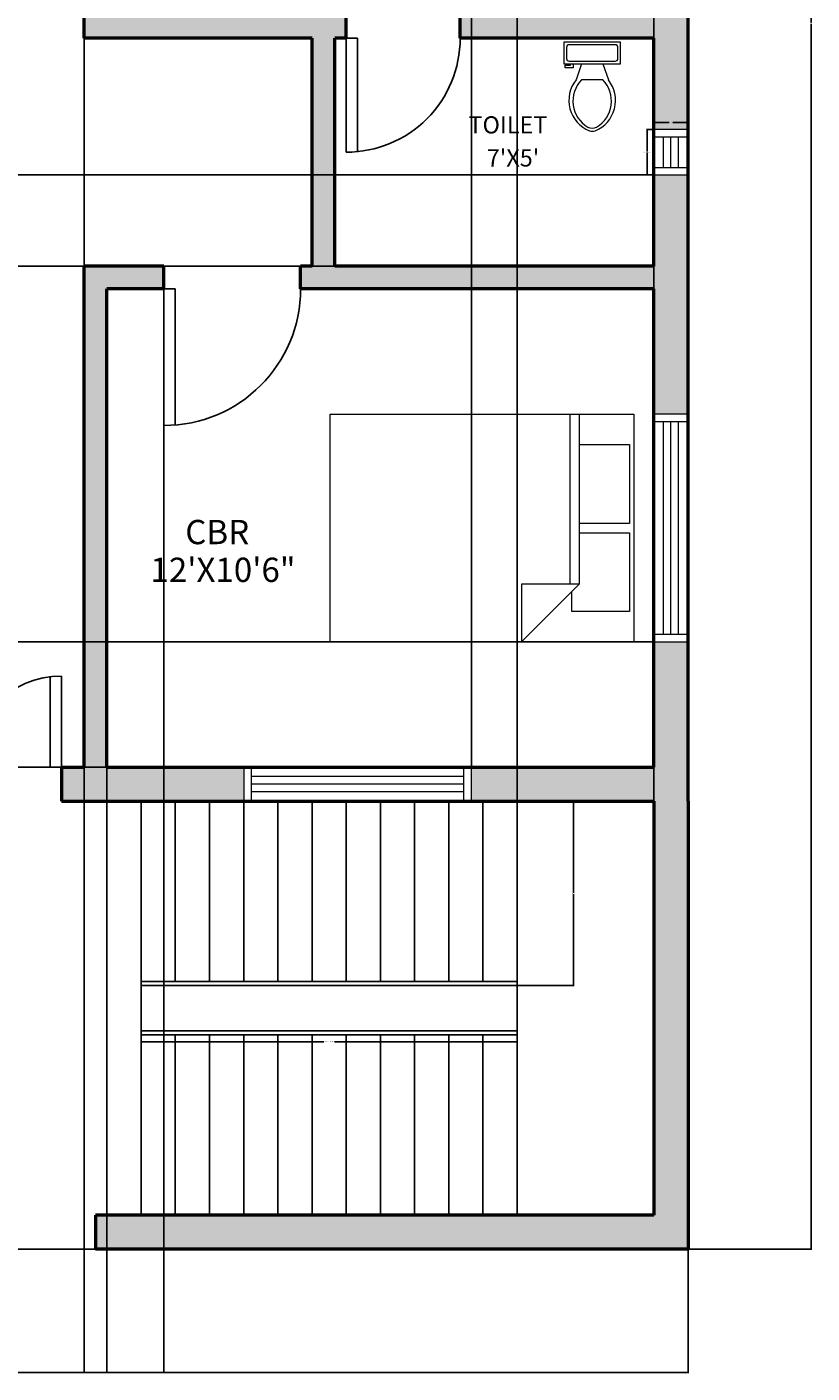
# Model space of a CAD drawing. Units: inches. Extents: x 96 to 522, y 502 to 1213.
# Tile 2 of 5: x 315 to 522, y 502 to 856. Entities that reach past the tile are written whole.
import ezdxf

# ---------------------------------------------------------------- set-up
doc = ezdxf.new("R2010")
doc.units = ezdxf.units.IN
doc.layers.get('Defpoints').update_dxf_attribs({"color": 90})
for name, color, linetype, lineweight in [('A-ANNO-DIMS', 2, 'Continuous', 18), ('A-AREA-IDEN', 7, 'Continuous', 25), ('A-DOOR', 3, 'Continuous', 25), ('A-FLOR', 7, 'Continuous', 25), ('A-FLOR-FIXT', 9, 'Continuous', 18), ('A-FLOR-STRS', 7, 'Continuous', 25), ('A-FURN', 8, 'Continuous', 18), ('A-GLAZ', 4, 'Continuous', 18), ('A-WALL', 7, 'Continuous', 50)]:
    doc.layers.add(name, color=color, linetype=linetype, lineweight=lineweight)
doc.layers.add('A-WALL-PATT', color=252, linetype='Continuous', lineweight=13, true_color=0x939598)
doc.styles.get("Standard").update_dxf_attribs({"font": 'arial.ttf'})
doc.dimstyles.get("Standard").update_dxf_attribs({"dimtxt": 0.18, "dimasz": 0.18, "dimexe": 0.18, "dimexo": 0.0625, "dimgap": 0.09, "dimtad": 0, "dimtih": 1, "dimtoh": 1, "dimdec": 4, "dimzin": 0, "dimdsep": 46, "dimtxsty": 'Standard', "dimcen": 0.09, "dimadec": 0, "dimazin": 0, "dimtfac": 1, "dimtdec": 4, "dimtofl": 0, "dimtmove": 0, "dimatfit": 3, "dimfxl": 1, "dimtolj": 1, "dimtzin": 0, "dimarcsym": 0})

# ---------------------------------------------------------------- blocks, each defined once
blk = doc.blocks.new('Bed - Queen')
for p, q in [((0, -80.00003), (0, 0)), ((0, 0), (59.99999, 0)), ((59.99999, 0), (59.99999, -80.00003)), ((7.99999, -1.2), (28.79998, -1.2)), ((7.99999, -14.4), (7.99999, -1.2)), ((28.79998, -1.2), (28.79998, -14.4)), ((31.19999, -1.2), (51.99999, -1.2)), ((31.19999, -14.4), (31.19999, -1.2)), ((51.99999, -1.2), (51.99999, -16.4)), ((0, -14.4), (44.8, -14.4)), ((44.8, -16.8), (0, -16.8)), ((59.99999, -29.6), (44.8, -14.4)), ((44.8, -14.4), (44.8, -29.6)), ((51.99999, -16.4), (46.79936, -16.4)), ((44.8, -29.6), (59.99999, -29.6)), ((59.99999, -80.00003), (0, -80.00003))]:
    blk.add_line(p, q)
blk = doc.blocks.new('Toilet - top')
for p, q in [((9.5, -6), (9.5, -2)), ((-10, -8.5), (-8, -8.5)), ((-10, -9.5), (-10, -8.5)), ((-7, -9.5), (-10, -9.5)), ((-8, -8.5), (-8, -8)), ((-7, -8), (-7, -9.5)), ((-4, -8), (-6, -14)), ((4, -8), (6, -14)), ((4, -14), (-4, -14))]:
    blk.add_line(p, q)
blk.add_lwpolyline([(10.5, -8), (10.5, 0), (-10.5, 0), (-10.5, -8)], close=True)
for points in [[(-9.5, -2), (-9.5, -6)], [(8.5, -1), (-8.5, -1)], [(-8.5, -7), (8.5, -7)]]:
    blk.add_lwpolyline(points)
for centre, radius, start, end in [((-8.62, -1.88), 0.884, 81.8699, 188.1301), ((8.62, -1.88), 0.884, 351.8699, 98.1301), ((-8.62, -6.12), 0.884, 171.8699, 278.1301), ((8.62, -6.12), 0.884, 261.8699, 8.1301), ((3.52, -21.58), 12.17, 141.4691, 247.9714), ((4.2, -21.82), 11.33, 136.3677, 238.9468), ((-3.52, -21.58), 12.17, 292.0284, 38.5307), ((-4.2, -21.82), 11.33, 301.053, 43.6321), ((0, -27.88), 4, 245.7318, 294.2682), ((0, -29), 4, 254.8605, 285.1395)]:
    blk.add_arc(centre, radius, start, end)
blk = doc.blocks.new('WIN-60IN')
for p, q in [((60, 9), (0, 9)), ((0, 9), (0, 0)), ((2, 9), (2, 0)), ((58, 0), (58, 9)), ((60, 0), (60, 9)), ((2, 6.5), (58, 6.5)), ((2, 4.5), (58, 4.5)), ((0, 0), (60, 0)), ((2, 2.5), (58, 2.5))]:
    blk.add_line(p, q)
blk = doc.blocks.new('WIN-12IN')
for p, q in [((0, 12), (0, 0)), ((9, 12), (0, 12)), ((9, 0), (9, 12)), ((9, 10), (0, 10)), ((2.5, 10), (2.5, 2)), ((4.5, 10), (4.5, 2)), ((6.5, 10), (6.5, 2)), ((0, 2), (9, 2)), ((0, 0), (9, 0))]:
    blk.add_line(p, q)
blk = doc.blocks.new('DOOR-SGL-36IN')
for p, q in [((36, 3), (0, 3)), ((0, 0), (0, 3)), ((36, 0), (0, 0))]:
    blk.add_line(p, q)
blk.add_arc((0, 0), 36, 0, 90)
blk = doc.blocks.new('DOOR-SGL-30IN')
for p, q in [((30, 30), (0, 30)), ((0, 30), (0, 27)), ((30, 27), (0, 27))]:
    blk.add_line(p, q)
blk.add_arc((0, 30), 30, 270, 0)
blk = doc.blocks.new('DOOR-DBL-48IN')
for p, q in [((0, 24), (0, 0)), ((3, 24), (3, 0)), ((45, 24), (45, 0)), ((48, 24), (48, 0)), ((0, 0), (3, 0)), ((48, 0), (45, 0))]:
    blk.add_line(p, q)
for centre, start, end in [((0, 0), 0, 90), ((48, 0), 90, 180)]:
    blk.add_arc(centre, 24, start, end)
blk = doc.blocks.new('STAIR-FLIGHT-11-TREAD')
for p, q in [((0, 48.5), (0, 0)), ((9, 48.5), (9, 1)), ((18, 48.5), (18, 1)), ((27, 48.5), (27, 1)), ((36, 48.5), (36, 1)), ((45, 48.5), (45, 1)), ((54, 48.5), (54, 1)), ((63, 48.5), (63, 1)), ((72, 48.5), (72, 1)), ((81, 48.5), (81, 1)), ((90, 48.5), (90, 1)), ((99, 48.5), (99, 1)), ((0, 1), (99, 1)), ((0, 0), (99, 0)), ((99, 0), (99, 1))]:
    blk.add_line(p, q)
blk = doc.blocks.new('*D19')
at = {"layer": 'A-ANNO-DIMS', "color": 0, "lineweight": -2, "transparency": 16777216}
for p, q in [((480.15, 829.25), (478.23, 829.25)), ((478.41, 829.07), (478.41, 823.43)), ((478.41, 817.43), (478.41, 823.07)), ((480.15, 817.25), (478.23, 817.25))]:
    blk.add_line(p, q, dxfattribs=at)
at = {"layer": 'A-ANNO-DIMS', "color": 0, "transparency": 16777216}
for points in [[(478.38, 829.07), (478.44, 829.07), (478.41, 829.25)], [(478.38, 817.43), (478.44, 817.43), (478.41, 817.25)]]:
    blk.add_solid(points, dxfattribs=at)
at = {"layer": 'Defpoints', "color": 0, "transparency": 16777216}
for p in [(480.21, 829.25), (478.41, 817.25), (480.21, 817.25)]:
    blk.add_point(p, dxfattribs=at)
at = {"layer": 'A-ANNO-DIMS', "color": 0, "transparency": 16777216, "insert": (478.41, 823.25), "char_height": 0.18, "attachment_point": 5}
blk.add_mtext('\\A1;WINDOW 12 TYP.', dxfattribs=at)
blk = doc.blocks.new('*D20')
at = {"layer": 'A-ANNO-DIMS', "color": 0, "lineweight": -2, "transparency": 16777216}
for p, q in [((480.21, 829.31), (480.21, 831.23)), ((480.39, 831.05), (484.25, 831.05)), ((489.03, 831.05), (485.17, 831.05)), ((489.21, 829.31), (489.21, 831.23))]:
    blk.add_line(p, q, dxfattribs=at)
at = {"layer": 'A-ANNO-DIMS', "color": 0, "transparency": 16777216}
for points in [[(480.39, 831.08), (480.39, 831.02), (480.21, 831.05)], [(489.03, 831.08), (489.03, 831.02), (489.21, 831.05)]]:
    blk.add_solid(points, dxfattribs=at)
at = {"layer": 'Defpoints', "color": 0, "transparency": 16777216}
for p in [(480.21, 831.05), (480.21, 829.25), (489.21, 829.25)]:
    blk.add_point(p, dxfattribs=at)
at = {"layer": 'A-ANNO-DIMS', "color": 0, "transparency": 16777216, "insert": (484.71, 831.05), "char_height": 0.18, "attachment_point": 5}
blk.add_mtext('\\A1;9 TYP.', dxfattribs=at)
blk = doc.blocks.new('*D31')
at = {"layer": 'A-ANNO-DIMS', "color": 0, "lineweight": -2, "transparency": 16777216}
for p, q in [((345.21, 603.69), (345.21, 588.72)), ((444.21, 603.69), (444.21, 588.72)), ((345.39, 588.9), (393.3, 588.9)), ((444.03, 588.9), (396.13, 588.9))]:
    blk.add_line(p, q, dxfattribs=at)
at = {"layer": 'A-ANNO-DIMS', "color": 0, "transparency": 16777216}
for points in [[(345.39, 588.93), (345.39, 588.87), (345.21, 588.9)], [(444.03, 588.93), (444.03, 588.87), (444.21, 588.9)]]:
    blk.add_solid(points, dxfattribs=at)
at = {"layer": 'Defpoints', "color": 0, "transparency": 16777216}
for p in [(345.21, 603.75), (444.21, 603.75), (444.21, 588.9)]:
    blk.add_point(p, dxfattribs=at)
at = {"layer": 'A-ANNO-DIMS', "color": 0, "transparency": 16777216, "insert": (394.71, 588.9), "char_height": 0.18, "attachment_point": 5}
blk.add_mtext('\\A1;STAIR FLIGHT 99 TYP.', dxfattribs=at)
blk = doc.blocks.new('*D32')
at = {"layer": 'A-ANNO-DIMS', "color": 0, "lineweight": -2, "transparency": 16777216}
for p, q in [((444.27, 652.25), (459.24, 652.25)), ((459.06, 652.07), (459.06, 628.18)), ((459.06, 603.93), (459.06, 627.82)), ((444.27, 603.75), (459.24, 603.75))]:
    blk.add_line(p, q, dxfattribs=at)
at = {"layer": 'A-ANNO-DIMS', "color": 0, "transparency": 16777216}
for points in [[(459.03, 652.07), (459.09, 652.07), (459.06, 652.25)], [(459.03, 603.93), (459.09, 603.93), (459.06, 603.75)]]:
    blk.add_solid(points, dxfattribs=at)
at = {"layer": 'Defpoints', "color": 0, "transparency": 16777216}
for p in [(444.21, 652.25), (459.06, 652.25), (444.21, 603.75)]:
    blk.add_point(p, dxfattribs=at)
at = {"layer": 'A-ANNO-DIMS', "color": 0, "transparency": 16777216, "insert": (459.06, 628), "char_height": 0.18, "attachment_point": 5}
blk.add_mtext('\\A1;49 TYP.', dxfattribs=at)
blk = doc.blocks.new('*D47')
at = {"layer": 'A-ANNO-DIMS', "color": 0, "lineweight": -2, "transparency": 16777216}
for p, q in [((129.21, 534.19), (129.21, 501.62)), ((489.21, 534.19), (489.21, 501.62)), ((129.39, 501.8), (308.92, 501.8)), ((489.03, 501.8), (309.5, 501.8))]:
    blk.add_line(p, q, dxfattribs=at)
at = {"layer": 'A-ANNO-DIMS', "color": 0, "transparency": 16777216}
for points in [[(129.39, 501.83), (129.39, 501.77), (129.21, 501.8)], [(489.03, 501.83), (489.03, 501.77), (489.21, 501.8)]]:
    blk.add_solid(points, dxfattribs=at)
at = {"layer": 'Defpoints', "color": 0, "transparency": 16777216}
for p in [(129.21, 534.25), (489.21, 534.25), (489.21, 501.8)]:
    blk.add_point(p, dxfattribs=at)
at = {"layer": 'A-ANNO-DIMS', "color": 0, "transparency": 16777216, "insert": (309.21, 501.8), "char_height": 0.18, "attachment_point": 5}
blk.add_mtext('\\A1;360', dxfattribs=at)
blk = doc.blocks.new('*D48')
at = {"layer": 'A-ANNO-DIMS', "color": 0, "lineweight": -2, "transparency": 16777216}
for p, q in [((335.27, 1180.25), (521.84, 1180.25)), ((521.66, 1180.07), (521.66, 857.43)), ((521.66, 534.43), (521.66, 857.07)), ((489.27, 534.25), (521.84, 534.25))]:
    blk.add_line(p, q, dxfattribs=at)
at = {"layer": 'A-ANNO-DIMS', "color": 0, "transparency": 16777216}
for points in [[(521.63, 1180.07), (521.69, 1180.07), (521.66, 1180.25)], [(521.63, 534.43), (521.69, 534.43), (521.66, 534.25)]]:
    blk.add_solid(points, dxfattribs=at)
at = {"layer": 'Defpoints', "color": 0, "transparency": 16777216}
for p in [(335.21, 1180.25), (521.66, 1180.25), (489.21, 534.25)]:
    blk.add_point(p, dxfattribs=at)
at = {"layer": 'A-ANNO-DIMS', "color": 0, "transparency": 16777216, "insert": (521.66, 857.25), "char_height": 0.18, "attachment_point": 5}
blk.add_mtext('\\A1;646', dxfattribs=at)
blk = doc.blocks.new('*D55')
at = {"layer": 'A-ANNO-DIMS', "color": 0, "lineweight": -2, "transparency": 16777216}
for p, q in [((432.21, 661.31), (432.21, 1212.88)), ((480.21, 661.31), (480.21, 1212.88)), ((432.39, 1212.7), (455.99, 1212.7)), ((480.03, 1212.7), (456.43, 1212.7))]:
    blk.add_line(p, q, dxfattribs=at)
at = {"layer": 'A-ANNO-DIMS', "color": 0, "transparency": 16777216}
for points in [[(432.39, 1212.73), (432.39, 1212.67), (432.21, 1212.7)], [(480.03, 1212.73), (480.03, 1212.67), (480.21, 1212.7)]]:
    blk.add_solid(points, dxfattribs=at)
at = {"layer": 'Defpoints', "color": 0, "transparency": 16777216}
for p in [(480.21, 1212.7), (432.21, 661.25), (480.21, 661.25)]:
    blk.add_point(p, dxfattribs=at)
at = {"layer": 'A-ANNO-DIMS', "color": 0, "transparency": 16777216, "insert": (456.21, 1212.7), "char_height": 0.18, "attachment_point": 5}
blk.add_mtext('\\A1;48', dxfattribs=at)
blk = doc.blocks.new('*D60')
at = {"layer": 'A-ANNO-DIMS', "color": 0, "lineweight": -2, "transparency": 16777216}
for p, q in [((480.15, 694.25), (96.58, 694.25)), ((96.76, 694.07), (96.76, 677.93)), ((96.76, 661.43), (96.76, 677.57)), ((480.15, 661.25), (96.58, 661.25))]:
    blk.add_line(p, q, dxfattribs=at)
at = {"layer": 'A-ANNO-DIMS', "color": 0, "transparency": 16777216}
for points in [[(96.73, 694.07), (96.79, 694.07), (96.76, 694.25)], [(96.73, 661.43), (96.79, 661.43), (96.76, 661.25)]]:
    blk.add_solid(points, dxfattribs=at)
at = {"layer": 'Defpoints', "color": 0, "transparency": 16777216}
for p in [(96.76, 694.25), (480.21, 694.25), (480.21, 661.25)]:
    blk.add_point(p, dxfattribs=at)
at = {"layer": 'A-ANNO-DIMS', "color": 0, "transparency": 16777216, "insert": (96.76, 677.75), "char_height": 0.18, "attachment_point": 5}
blk.add_mtext('\\A1;33', dxfattribs=at)
blk = doc.blocks.new('*D61')
at = {"layer": 'A-ANNO-DIMS', "color": 0, "lineweight": -2, "transparency": 16777216}
for p, q in [((480.15, 817.25), (96.58, 817.25)), ((96.76, 817.07), (96.76, 805.43)), ((96.76, 793.43), (96.76, 805.07)), ((480.15, 793.25), (96.58, 793.25))]:
    blk.add_line(p, q, dxfattribs=at)
at = {"layer": 'A-ANNO-DIMS', "color": 0, "transparency": 16777216}
for points in [[(96.73, 817.07), (96.79, 817.07), (96.76, 817.25)], [(96.73, 793.43), (96.79, 793.43), (96.76, 793.25)]]:
    blk.add_solid(points, dxfattribs=at)
at = {"layer": 'Defpoints', "color": 0, "transparency": 16777216}
for p in [(96.76, 817.25), (480.21, 817.25), (480.21, 793.25)]:
    blk.add_point(p, dxfattribs=at)
at = {"layer": 'A-ANNO-DIMS', "color": 0, "transparency": 16777216, "insert": (96.76, 805.25), "char_height": 0.18, "attachment_point": 5}
blk.add_mtext('\\A1;24', dxfattribs=at)
blk = doc.blocks.new('*D65')
at = {"layer": 'A-ANNO-DIMS', "color": 0, "lineweight": -2, "transparency": 16777216}
for p, q in [((444.21, 543.31), (444.21, 1212.88)), ((480.21, 543.31), (480.21, 1212.88)), ((444.39, 1212.7), (461.99, 1212.7)), ((480.03, 1212.7), (462.43, 1212.7))]:
    blk.add_line(p, q, dxfattribs=at)
at = {"layer": 'A-ANNO-DIMS', "color": 0, "transparency": 16777216}
for points in [[(444.39, 1212.73), (444.39, 1212.67), (444.21, 1212.7)], [(480.03, 1212.73), (480.03, 1212.67), (480.21, 1212.7)]]:
    blk.add_solid(points, dxfattribs=at)
at = {"layer": 'Defpoints', "color": 0, "transparency": 16777216}
for p in [(480.21, 1212.7), (444.21, 543.25), (480.21, 543.25)]:
    blk.add_point(p, dxfattribs=at)
at = {"layer": 'A-ANNO-DIMS', "color": 0, "transparency": 16777216, "insert": (462.21, 1212.7), "char_height": 0.18, "attachment_point": 5}
blk.add_mtext('\\A1;36', dxfattribs=at)
blk = doc.blocks.new('*D66')
at = {"layer": 'A-ANNO-DIMS', "color": 0, "lineweight": -2, "transparency": 16777216}
for p, q in [((330.21, 1033.19), (330.21, 501.62)), ((276.21, 997.19), (276.21, 501.62)), ((276.39, 501.8), (302.99, 501.8)), ((330.03, 501.8), (303.43, 501.8))]:
    blk.add_line(p, q, dxfattribs=at)
at = {"layer": 'A-ANNO-DIMS', "color": 0, "transparency": 16777216}
for points in [[(276.39, 501.83), (276.39, 501.77), (276.21, 501.8)], [(330.03, 501.83), (330.03, 501.77), (330.21, 501.8)]]:
    blk.add_solid(points, dxfattribs=at)
at = {"layer": 'Defpoints', "color": 0, "transparency": 16777216}
for p in [(330.21, 1033.25), (276.21, 997.25), (330.21, 501.8)]:
    blk.add_point(p, dxfattribs=at)
at = {"layer": 'A-ANNO-DIMS', "color": 0, "transparency": 16777216, "insert": (303.21, 501.8), "char_height": 0.18, "attachment_point": 5}
blk.add_mtext('\\A1;54', dxfattribs=at)
blk = doc.blocks.new('*D70')
at = {"layer": 'A-ANNO-DIMS', "color": 0, "lineweight": -2, "transparency": 16777216}
for p, q in [((336.21, 787.19), (336.21, 501.62)), ((351.21, 787.19), (351.21, 501.62)), ((336.39, 501.8), (343.5, 501.8)), ((351.03, 501.8), (343.92, 501.8))]:
    blk.add_line(p, q, dxfattribs=at)
at = {"layer": 'A-ANNO-DIMS', "color": 0, "transparency": 16777216}
for points in [[(336.39, 501.83), (336.39, 501.77), (336.21, 501.8)], [(351.03, 501.83), (351.03, 501.77), (351.21, 501.8)]]:
    blk.add_solid(points, dxfattribs=at)
at = {"layer": 'Defpoints', "color": 0, "transparency": 16777216}
for p in [(336.21, 787.25), (351.21, 787.25), (351.21, 501.8)]:
    blk.add_point(p, dxfattribs=at)
at = {"layer": 'A-ANNO-DIMS', "color": 0, "transparency": 16777216, "insert": (343.71, 501.8), "char_height": 0.18, "attachment_point": 5}
blk.add_mtext('\\A1;15', dxfattribs=at)

msp = doc.modelspace()

# ---------------------------------------------------------------- hatches: boundary and pattern name
at = {"layer": 'A-WALL-PATT'}
h = msp.add_hatch(color=256, dxfattribs=at)
h.dxf.hatch_style = 1
h.paths.add_polyline_path([(174.2111, 1156.2511), (129.2111, 1156.2511), (129.2111, 1105.2511), (138.2111, 1105.2511), (138.2111, 1147.2511), (174.2111, 1147.2511)])
h.paths.add_polyline_path([(287.2111, 1156.2511), (234.2111, 1156.2511), (234.2111, 1147.2511), (270.2111, 1147.2511), (270.2111, 1003.2511), (267.2111, 1003.2511), (267.2111, 997.2511), (276.2111, 997.2511), (276.2111, 1147.2511), (287.2111, 1147.2511)])
h.paths.add_polyline_path([(342.2111, 1156.2511), (335.2111, 1156.2511), (335.2111, 1147.2511), (338.2111, 1147.2511), (338.2111, 1081.2511), (342.2111, 1081.2511), (342.2111, 1147.2511)])
h.paths.add_polyline_path([(489.2111, 1156.2511), (402.2111, 1156.2511), (402.2111, 1147.2511), (402.2111, 1141.2511), (408.2111, 1141.2511), (408.2111, 1147.2511), (480.2111, 1147.2511), (480.2111, 1123.2511), (489.2111, 1123.2511)])
h.paths.add_polyline_path([(489.2111, 1111.2511), (480.2111, 1111.2511), (480.2111, 1087.2511), (408.2111, 1087.2511), (408.2111, 1111.2511), (402.2111, 1111.2511), (402.2111, 1066.2511), (408.2111, 1066.2511), (408.2111, 1081.2511), (480.2111, 1081.2511), (480.2111, 1063.2511), (489.2111, 1063.2511)])
h.paths.add_polyline_path([(489.2111, 1051.2511), (480.2111, 1051.2511), (480.2111, 1033.2511), (408.2111, 1033.2511), (408.2111, 1036.2511), (402.2111, 1036.2511), (402.2111, 1033.2511), (338.2111, 1033.2511), (330.2111, 1033.2511), (330.2111, 923.2511), (336.2111, 923.2511), (336.2111, 1027.2511), (338.2111, 1027.2511), (402.2111, 1027.2511), (480.2111, 1027.2511), (480.2111, 973.2511), (489.2111, 973.2511)])
h.paths.add_polyline_path([(489.2111, 913.2511), (480.2111, 913.2511), (480.2111, 859.2511), (429.2111, 859.2511), (429.2111, 853.2511), (480.2111, 853.2511), (480.2111, 829.2511), (489.2111, 829.2511)])
h.paths.add_polyline_path([(489.2111, 817.2511), (480.2111, 817.2511), (480.2111, 793.2511), (402.2111, 793.2511), (396.2111, 793.2511), (396.2111, 853.2511), (399.2111, 853.2511), (399.2111, 859.2511), (338.2111, 859.2511), (336.2111, 859.2511), (336.2111, 877.2511), (336.2111, 883.2511), (336.2111, 887.2511), (330.2111, 887.2511), (330.2111, 883.2511), (326.2111, 883.2511), (326.2111, 877.2511), (330.2111, 877.2511), (330.2111, 853.2511), (338.2111, 853.2511), (390.2111, 853.2511), (390.2111, 793.2511), (387.2111, 793.2511), (387.2111, 787.2511), (402.2111, 787.2511), (480.2111, 787.2511), (480.2111, 754.2511), (489.2111, 754.2511)])
h.paths.add_polyline_path([(489.2111, 694.2511), (480.2111, 694.2511), (480.2111, 661.2511), (432.2111, 661.2511), (432.2111, 652.2511), (480.2111, 652.2511), (480.2111, 543.2511), (333.2111, 543.2511), (333.2111, 534.2511), (489.2111, 534.2511), (489.2111, 652.2511)])
h.paths.add_polyline_path([(372.2111, 661.2511), (336.2111, 661.2511), (336.2111, 787.2511), (338.2111, 787.2511), (351.2111, 787.2511), (351.2111, 793.2511), (338.2111, 793.2511), (330.2111, 793.2511), (330.2111, 661.2511), (324.2111, 661.2511), (324.2111, 652.2511), (372.2111, 652.2511)])
h.paths.add_polyline_path([(138.2111, 680.6946), (129.2111, 680.6946), (129.2111, 652.2511), (177.2111, 652.2511), (177.2111, 661.2511), (138.2111, 661.2511)])
h.paths.add_polyline_path([(276.2111, 661.2511), (237.2111, 661.2511), (237.2111, 652.2511), (276.2111, 652.2511)])
h.paths.add_polyline_path([(138.2111, 803.1393), (129.2111, 803.1393), (129.2111, 740.6946), (138.2111, 740.6946)])
h.paths.add_polyline_path([(138.2111, 907.2511), (129.2111, 907.2511), (129.2111, 863.1393), (138.2111, 863.1393), (138.2111, 877.2511), (276.2111, 877.2511), (276.2111, 883.2511), (204.2111, 883.2511), (204.2111, 886.2511), (198.2111, 886.2511), (198.2111, 883.2511), (138.2111, 883.2511)])
h.paths.add_polyline_path([(138.2111, 943.2511), (198.2111, 943.2511), (198.2111, 916.2511), (204.2111, 916.2511), (204.2111, 949.2511), (138.2111, 949.2511), (138.2111, 997.2511), (231.2111, 997.2511), (231.2111, 1003.2511), (138.2111, 1003.2511), (138.2111, 1045.2511), (129.2111, 1045.2511), (129.2111, 919.2511), (138.2111, 919.2511)])

# ---------------------------------------------------------------- linework, layer by layer
at = {"layer": 'A-FLOR'}
msp.add_line((129.2111, 534.2511), (333.2111, 534.2511), dxfattribs=at)
at = {"layer": 'A-WALL'}
for p, q in [((330.2111, 853.2511), (330.2111, 877.2511)), ((399.2111, 853.2511), (399.2111, 859.2511)), ((429.2111, 853.2511), (429.2111, 859.2511)), ((338.2111, 853.2511), (330.2111, 853.2511)), ((390.2111, 853.2511), (338.2111, 853.2511)), ((390.2111, 793.2511), (390.2111, 853.2511)), ((399.2111, 853.2511), (396.2111, 853.2511)), ((396.2111, 793.2511), (396.2111, 853.2511)), ((480.2111, 853.2511), (429.2111, 853.2511)), ((480.2111, 793.2511), (480.2111, 853.2511)), ((330.2111, 661.2511), (330.2111, 793.2511)), ((338.2111, 793.2511), (330.2111, 793.2511)), ((351.2111, 793.2511), (338.2111, 793.2511)), ((351.2111, 787.2511), (351.2111, 793.2511)), ((387.2111, 787.2511), (387.2111, 793.2511)), ((390.2111, 793.2511), (387.2111, 793.2511)), ((402.2111, 793.2511), (396.2111, 793.2511)), ((480.2111, 793.2511), (402.2111, 793.2511)), ((336.2111, 661.2511), (336.2111, 787.2511)), ((338.2111, 787.2511), (336.2111, 787.2511)), ((351.2111, 787.2511), (338.2111, 787.2511)), ((402.2111, 787.2511), (387.2111, 787.2511)), ((480.2111, 787.2511), (402.2111, 787.2511)), ((480.2111, 661.2511), (480.2111, 787.2511)), ((324.2111, 661.2511), (324.2111, 652.2511)), ((324.2111, 661.2511), (330.2111, 661.2511)), ((336.2111, 661.2511), (480.2111, 661.2511)), ((480.2111, 652.2511), (480.2111, 543.2511)), ((489.2111, 652.2511), (489.2111, 534.2511)), ((333.2111, 543.2511), (333.2111, 534.2511)), ((480.2111, 543.2511), (333.2111, 543.2511)), ((489.2111, 534.2511), (333.2111, 534.2511))]:
    msp.add_line(p, q, dxfattribs=at)
for points in [[(489.2111, 652.2511), (489.2111, 1156.2511), (335.2111, 1156.2511)], [(324.2111, 652.2511), (480.2111, 652.2511)]]:
    msp.add_lwpolyline(points, dxfattribs=at)

# ---------------------------------------------------------------- block references
at = {"layer": 'A-DOOR', "extrusion": (0, 0, -1), "zscale": -1, "rotation": 270.0000000000007}
msp.add_blockref('DOOR-SGL-30IN', (-429.2111, 853.2511), dxfattribs=at)
at = {"layer": 'A-DOOR', "rotation": 269.9999999999998}
msp.add_blockref('DOOR-SGL-36IN', (351.2111, 787.2511), dxfattribs=at)
at = {"layer": 'A-DOOR'}
msp.add_blockref('DOOR-DBL-48IN', (276.2111, 661.2511), dxfattribs=at)
at = {"layer": 'A-FLOR-FIXT', "xscale": 0.7100067742046297, "yscale": 0.7100067742046297, "zscale": 0.7100067742046297}
msp.add_blockref('Toilet - top', (463.9746, 852.2313), dxfattribs=at)
at = {"layer": 'A-FLOR-STRS'}
msp.add_blockref('STAIR-FLIGHT-11-TREAD', (345.2111, 603.7511), dxfattribs=at)
at = {"layer": 'A-FLOR-STRS', "extrusion": (0, 0, -1), "zscale": -1, "rotation": 180}
msp.add_blockref('STAIR-FLIGHT-11-TREAD', (-345.2111, 591.7511), dxfattribs=at)
at = {"layer": 'A-FURN', "rotation": 270}
msp.add_blockref('Bed - Queen', (474.9701, 754.2162), dxfattribs=at)
at = {"layer": 'A-GLAZ'}
for name, p, rotation in [('WIN-12IN', (489.2111, 829.2511), 180), ('WIN-60IN', (489.2111, 694.2511), 89.99999999999974), ('WIN-60IN', (432.2111, 661.2511), 180)]:
    msp.add_blockref(name, p, dxfattribs=dict(at, rotation=rotation))

# ---------------------------------------------------------------- texts
at = {"layer": 'A-AREA-IDEN', "attachment_point": 1}
for s, width, gutter_width, insert, char_height in [('TOILET', 24.813541, 22.6256, (431.4025, 832.7088), 4.52513), ("7'X5'", 24.813541, 22.6256, (436.2164, 824.0022), 4.52513), ('CBR', 35.064426, 31.9727, (356.8247, 726.3827), 6.39453), ('12\'X10\'6"', 35.064426, 31.9727, (347.6675, 716.4289), 6.39453)]:
    msp.add_mtext_dynamic_manual_height_columns(s, width=width, gutter_width=gutter_width, heights=[0], dxfattribs=dict(at, insert=insert, char_height=char_height))

# ---------------------------------------------------------------- dimensions: what is measured, and where the dimension line sits
at = {"layer": 'A-ANNO-DIMS'}
for base, p1, p2, picture, middle in [((480.2111, 1212.7011), (432.2111, 661.2511), (480.2111, 661.2511), '*D55', (456.2111, 1212.7011)), ((480.2111, 1212.7011), (444.2111, 543.2511), (480.2111, 543.2511), '*D65', (462.2111, 1212.7011)), ((330.2111, 501.8011), (276.2111, 997.2511), (330.2111, 1033.2511), '*D66', (303.2111, 501.8011)), ((351.2111, 501.8011), (336.2111, 787.2511), (351.2111, 787.2511), '*D70', (343.7111, 501.8011)), ((489.2111, 501.8011), (129.2111, 534.2511), (489.2111, 534.2511), '*D47', (309.2111, 501.8011))]:
    dim = msp.add_linear_dim(base=base, p1=p1, p2=p2, dimstyle='Standard', override={"dimdec": 0, "dimlfac": 1, "dimrnd": 0, "dimzin": 0, "dimdsep": 46, "dimlunit": 2}, dxfattribs=at)
    dim.commit()
    dim.dimension.update_dxf_attribs({"geometry": picture, "text_midpoint": middle})
for base, p1, p2, picture, middle in [((521.6611, 1180.2511), (489.2111, 534.2511), (335.2111, 1180.2511), '*D48', (521.6611, 857.2511)), ((96.7611, 817.2511), (480.2111, 793.2511), (480.2111, 817.2511), '*D61', (96.7611, 805.2511)), ((96.7611, 694.2511), (480.2111, 661.2511), (480.2111, 694.2511), '*D60', (96.7611, 677.7511))]:
    dim = msp.add_linear_dim(base=base, p1=p1, p2=p2, angle=90, dimstyle='Standard', override={"dimdec": 0, "dimlfac": 1, "dimrnd": 0, "dimzin": 0, "dimdsep": 46, "dimlunit": 2}, dxfattribs=at)
    dim.commit()
    dim.dimension.update_dxf_attribs({"geometry": picture, "text_midpoint": middle})
for base, p1, p2, angle, text, picture, middle in [((480.2111, 831.0511), (489.2111, 829.2511), (480.2111, 829.2511), 180, '<> TYP.', '*D20', (484.7111, 831.0511)), ((478.4111, 817.2511), (480.2111, 829.2511), (480.2111, 817.2511), 270, 'WINDOW <> TYP.', '*D19', (478.4111, 823.2511)), ((459.0610874258, 652.2510824343), (444.2110874258, 603.7510824343), (444.2110874258, 652.2510824343), 90, '<> TYP.', '*D32', (459.0610874258, 628.0010824343))]:
    dim = msp.add_linear_dim(base=base, p1=p1, p2=p2, angle=angle, text=text, dimstyle='Standard', override={"dimdec": 0, "dimlfac": 1, "dimrnd": 0, "dimzin": 0, "dimdsep": 46, "dimlunit": 2}, dxfattribs=at)
    dim.commit()
    dim.dimension.update_dxf_attribs({"geometry": picture, "text_midpoint": middle})
dim = msp.add_linear_dim(base=(444.2111, 588.9011), p1=(345.2111, 603.7511), p2=(444.2111, 603.7511), text='STAIR FLIGHT <> TYP.', dimstyle='Standard', override={"dimdec": 0, "dimlfac": 1, "dimrnd": 0, "dimzin": 0, "dimdsep": 46, "dimlunit": 2}, dxfattribs=at)
dim.commit()
dim.dimension.update_dxf_attribs({"geometry": '*D31', "text_midpoint": (394.7111, 588.9011)})

doc.saveas('drawing.dxf')
